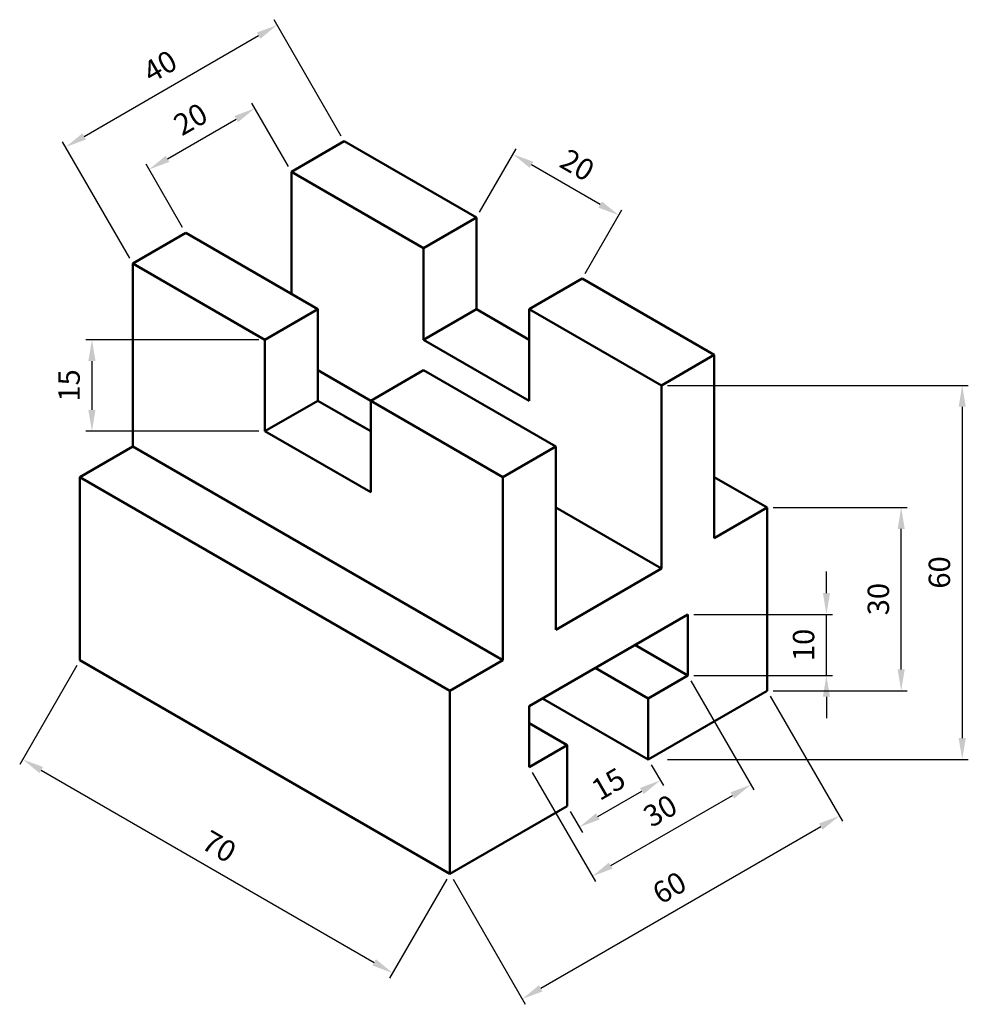
# Model space of a CAD drawing. Units: millimetres. Extents: x 130 to 285, y 54 to 215.
import ezdxf

# ---------------------------------------------------------------- set-up
doc = ezdxf.new("R2010")
doc.units = ezdxf.units.MM
doc.layers.add('M-DIMS', color=3, linetype='Continuous', lineweight=25)
doc.layers.add('M-OUTL', color=7, linetype='Continuous', lineweight=50)
doc.styles.get("Standard").update_dxf_attribs({"font": 'arial.ttf'})
doc.dimstyles.new('AM_ISO$0', dxfattribs={"dimtxt": 3.5, "dimasz": 3.5, "dimexe": 1, "dimexo": 1, "dimgap": 1.5, "dimtad": 1, "dimdsep": 46, "dimtxsty": 'Standard', "dimcen": 0, "dimclrd": 256, "dimclre": 256, "dimclrt": 3, "dimadec": 0, "dimazin": 2, "dimtp": 0.1, "dimtm": 0.1, "dimtfac": 0.71, "dimtmove": 0, "dimatfit": 3, "dimfxl": 1, "dimlwd": -1, "dimlwe": -1, "dimarcsym": 1})

# ---------------------------------------------------------------- blocks, each defined once
blk = doc.blocks.new('*D2')
at = {"layer": 'Defpoints', "color": 0, "transparency": 16777216}
for p in [(239.4, 117.98), (262.11, 117.98), (239.4, 107.98)]:
    blk.add_point(p, dxfattribs=at)
at = {"layer": 'M-DIMS', "color": 0, "linetype": 'ByBlock', "transparency": 16777216}
for p, q in [((262.11, 121.48), (262.11, 124.98)), ((240.4, 117.98), (263.11, 117.98)), ((262.11, 107.98), (262.11, 117.98)), ((240.4, 107.98), (263.11, 107.98)), ((262.11, 104.48), (262.11, 100.98))]:
    blk.add_line(p, q, dxfattribs=at)
at = {"layer": 'M-DIMS', "color": 0, "transparency": 16777216}
for points in [[(261.53, 121.48), (262.69, 121.48), (262.11, 117.98)], [(261.53, 104.48), (262.69, 104.48), (262.11, 107.98)]]:
    blk.add_solid(points, dxfattribs=at)
at = {"layer": 'M-DIMS', "color": 0, "transparency": 16777216, "insert": (258.82, 112.98), "char_height": 3.5, "attachment_point": 5, "rotation": 90}
blk.add_mtext('10', dxfattribs=at)
blk = doc.blocks.new('*D3')
at = {"layer": 'Defpoints', "color": 0, "transparency": 16777216}
for p in [(252.39, 135.48), (274.36, 135.48), (252.39, 105.48)]:
    blk.add_point(p, dxfattribs=at)
at = {"layer": 'M-DIMS', "color": 0, "linetype": 'ByBlock', "transparency": 16777216}
for p, q in [((253.39, 135.48), (275.36, 135.48)), ((274.36, 108.98), (274.36, 131.98)), ((253.39, 105.48), (275.36, 105.48))]:
    blk.add_line(p, q, dxfattribs=at)
at = {"layer": 'M-DIMS', "color": 0, "transparency": 16777216}
for points in [[(273.77, 131.98), (274.94, 131.98), (274.36, 135.48)], [(273.77, 108.98), (274.94, 108.98), (274.36, 105.48)]]:
    blk.add_solid(points, dxfattribs=at)
at = {"layer": 'M-DIMS', "color": 0, "transparency": 16777216, "insert": (271.07, 120.48), "char_height": 3.5, "attachment_point": 5, "rotation": 90}
blk.add_mtext('30', dxfattribs=at)
blk = doc.blocks.new('*D4')
at = {"layer": 'Defpoints', "color": 0, "transparency": 16777216}
for p in [(235.07, 155.48), (235.07, 94.23), (284.36, 94.23)]:
    blk.add_point(p, dxfattribs=at)
at = {"layer": 'M-DIMS', "color": 0, "linetype": 'ByBlock', "transparency": 16777216}
for p, q in [((236.07, 155.48), (285.36, 155.48)), ((284.36, 151.98), (284.36, 97.73)), ((236.07, 94.23), (285.36, 94.23))]:
    blk.add_line(p, q, dxfattribs=at)
at = {"layer": 'M-DIMS', "color": 0, "transparency": 16777216}
for points in [[(283.77, 151.98), (284.94, 151.98), (284.36, 155.48)], [(283.77, 97.73), (284.94, 97.73), (284.36, 94.23)]]:
    blk.add_solid(points, dxfattribs=at)
at = {"layer": 'M-DIMS', "color": 0, "transparency": 16777216, "insert": (281.07, 124.85), "char_height": 3.5, "attachment_point": 5, "rotation": 90}
blk.add_mtext('60', dxfattribs=at)
blk = doc.blocks.new('*D5')
at = {"layer": 'Defpoints', "color": 0, "transparency": 16777216}
for p in [(210.76, 193.37), (204.76, 182.98), (222.08, 172.98)]:
    blk.add_point(p, dxfattribs=at)
at = {"layer": 'M-DIMS', "color": 0, "linetype": 'ByBlock', "transparency": 16777216}
for p, q in [((205.26, 183.84), (211.26, 194.23)), ((225.05, 185.12), (213.79, 191.62)), ((222.58, 173.84), (228.58, 184.23))]:
    blk.add_line(p, q, dxfattribs=at)
at = {"layer": 'M-DIMS', "color": 0, "transparency": 16777216}
for points in [[(214.08, 192.12), (213.5, 191.11), (210.76, 193.37)], [(225.34, 185.62), (224.76, 184.61), (228.08, 183.37)]]:
    blk.add_solid(points, dxfattribs=at)
at = {"layer": 'M-DIMS', "color": 0, "transparency": 16777216, "insert": (221.07, 191.21), "char_height": 3.5, "attachment_point": 5, "rotation": 330}
blk.add_mtext('20', dxfattribs=at)
blk = doc.blocks.new('*D6')
at = {"layer": 'Defpoints', "color": 0, "transparency": 16777216}
for p in [(168.45, 200.87), (174.45, 190.48), (157.13, 180.48)]:
    blk.add_point(p, dxfattribs=at)
at = {"layer": 'M-DIMS', "color": 0, "linetype": 'ByBlock', "transparency": 16777216}
for p, q in [((173.95, 191.34), (167.95, 201.73)), ((154.16, 192.62), (165.42, 199.12)), ((156.63, 181.34), (150.63, 191.73))]:
    blk.add_line(p, q, dxfattribs=at)
at = {"layer": 'M-DIMS', "color": 0, "transparency": 16777216}
for points in [[(165.13, 199.62), (165.71, 198.61), (168.45, 200.87)], [(153.87, 193.12), (154.45, 192.11), (151.13, 190.87)]]:
    blk.add_solid(points, dxfattribs=at)
at = {"layer": 'M-DIMS', "color": 0, "transparency": 16777216, "insert": (158.15, 198.71), "char_height": 3.5, "attachment_point": 5, "rotation": 30}
blk.add_mtext('20', dxfattribs=at)
blk = doc.blocks.new('*D7')
at = {"layer": 'Defpoints', "color": 0, "transparency": 16777216}
for p in [(172.11, 214.53), (183.11, 195.48), (148.47, 175.48)]:
    blk.add_point(p, dxfattribs=at)
at = {"layer": 'M-DIMS', "color": 0, "linetype": 'ByBlock', "transparency": 16777216}
for p, q in [((182.61, 196.34), (171.61, 215.39)), ((140.5, 196.28), (169.08, 212.78)), ((147.97, 176.34), (136.97, 195.39))]:
    blk.add_line(p, q, dxfattribs=at)
at = {"layer": 'M-DIMS', "color": 0, "transparency": 16777216}
for points in [[(168.79, 213.28), (169.37, 212.27), (172.11, 214.53)], [(140.21, 196.78), (140.79, 195.77), (137.47, 194.53)]]:
    blk.add_solid(points, dxfattribs=at)
at = {"layer": 'M-DIMS', "color": 0, "transparency": 16777216, "insert": (153.15, 207.37), "char_height": 3.5, "attachment_point": 5, "rotation": 30}
blk.add_mtext('40', dxfattribs=at)
blk = doc.blocks.new('*D8')
at = {"layer": 'Defpoints', "color": 0, "transparency": 16777216}
for p in [(170.12, 162.98), (141.77, 147.98), (170.12, 147.98)]:
    blk.add_point(p, dxfattribs=at)
at = {"layer": 'M-DIMS', "color": 0, "linetype": 'ByBlock', "transparency": 16777216}
for p, q in [((169.12, 162.98), (140.77, 162.98)), ((141.77, 159.48), (141.77, 151.48)), ((169.12, 147.98), (140.77, 147.98))]:
    blk.add_line(p, q, dxfattribs=at)
at = {"layer": 'M-DIMS', "color": 0, "transparency": 16777216}
for points in [[(141.18, 159.48), (142.35, 159.48), (141.77, 162.98)], [(141.18, 151.48), (142.35, 151.48), (141.77, 147.98)]]:
    blk.add_solid(points, dxfattribs=at)
at = {"layer": 'M-DIMS', "color": 0, "transparency": 16777216, "insert": (138.48, 155.48), "char_height": 3.5, "attachment_point": 5, "rotation": 90}
blk.add_mtext('15', dxfattribs=at)
blk = doc.blocks.new('*D9')
at = {"layer": 'Defpoints', "color": 0, "transparency": 16777216}
for p in [(139.81, 110.48), (200.43, 75.48), (191.05, 59.23)]:
    blk.add_point(p, dxfattribs=at)
at = {"layer": 'M-DIMS', "color": 0, "linetype": 'ByBlock', "transparency": 16777216}
for p, q in [((139.31, 109.61), (129.93, 93.37)), ((133.46, 92.48), (188.02, 60.98)), ((199.93, 74.61), (190.55, 58.37))]:
    blk.add_line(p, q, dxfattribs=at)
at = {"layer": 'M-DIMS', "color": 0, "transparency": 16777216}
for points in [[(133.75, 92.99), (133.17, 91.98), (130.43, 94.23)], [(188.31, 61.49), (187.73, 60.48), (191.05, 59.23)]]:
    blk.add_solid(points, dxfattribs=at)
at = {"layer": 'M-DIMS', "color": 0, "transparency": 16777216, "insert": (162.39, 79.58), "char_height": 3.5, "attachment_point": 5, "rotation": 330}
blk.add_mtext('70', dxfattribs=at)
blk = doc.blocks.new('*D10')
at = {"layer": 'Defpoints', "color": 0, "transparency": 16777216}
for p in [(232.91, 94.23), (234.89, 90.8), (219.64, 86.57)]:
    blk.add_point(p, dxfattribs=at)
at = {"layer": 'M-DIMS', "color": 0, "linetype": 'ByBlock', "transparency": 16777216}
for p, q in [((233.41, 93.36), (235.39, 89.93)), ((224.65, 84.89), (231.85, 89.05)), ((220.14, 85.7), (222.12, 82.28))]:
    blk.add_line(p, q, dxfattribs=at)
at = {"layer": 'M-DIMS', "color": 0, "transparency": 16777216}
for points in [[(231.56, 89.55), (232.15, 88.54), (234.89, 90.8)], [(224.36, 85.4), (224.95, 84.39), (221.62, 83.14)]]:
    blk.add_solid(points, dxfattribs=at)
at = {"layer": 'M-DIMS', "color": 0, "transparency": 16777216, "insert": (226.61, 89.82), "char_height": 3.5, "attachment_point": 5, "rotation": 30}
blk.add_mtext('15', dxfattribs=at)
blk = doc.blocks.new('*D11')
at = {"layer": 'Defpoints', "color": 0, "transparency": 16777216}
for p in [(239.4, 107.98), (213.42, 92.98), (249.73, 90.08)]:
    blk.add_point(p, dxfattribs=at)
at = {"layer": 'M-DIMS', "color": 0, "linetype": 'ByBlock', "transparency": 16777216}
for p, q in [((239.9, 107.11), (250.23, 89.22)), ((213.92, 92.11), (224.25, 74.22)), ((226.78, 76.83), (246.7, 88.33))]:
    blk.add_line(p, q, dxfattribs=at)
at = {"layer": 'M-DIMS', "color": 0, "transparency": 16777216}
for points in [[(246.41, 88.84), (246.99, 87.83), (249.73, 90.08)], [(226.49, 77.34), (227.07, 76.33), (223.75, 75.08)]]:
    blk.add_solid(points, dxfattribs=at)
at = {"layer": 'M-DIMS', "color": 0, "transparency": 16777216, "insert": (235.1, 85.43), "char_height": 3.5, "attachment_point": 5, "rotation": 30}
blk.add_mtext('30', dxfattribs=at)
blk = doc.blocks.new('*D12')
at = {"layer": 'Defpoints', "color": 0, "transparency": 16777216}
for p in [(252.39, 105.48), (264.23, 84.98), (200.43, 75.48)]:
    blk.add_point(p, dxfattribs=at)
at = {"layer": 'M-DIMS', "color": 0, "linetype": 'ByBlock', "transparency": 16777216}
for p, q in [((252.89, 104.61), (264.73, 84.11)), ((215.3, 56.73), (261.2, 83.23)), ((200.93, 74.61), (212.77, 54.11))]:
    blk.add_line(p, q, dxfattribs=at)
at = {"layer": 'M-DIMS', "color": 0, "transparency": 16777216}
for points in [[(260.9, 83.73), (261.49, 82.72), (264.23, 84.98)], [(215, 57.23), (215.59, 56.22), (212.27, 54.98)]]:
    blk.add_solid(points, dxfattribs=at)
at = {"layer": 'M-DIMS', "color": 0, "transparency": 16777216, "insert": (236.6, 72.83), "char_height": 3.5, "attachment_point": 5, "rotation": 30}
blk.add_mtext('60', dxfattribs=at)

msp = doc.modelspace()

# ---------------------------------------------------------------- linework, layer by layer
at = {"layer": 'M-OUTL'}
for p, q in [((174.451, 190.475), (183.111, 195.475)), ((183.111, 195.475), (204.762, 182.975)), ((174.451, 190.475), (196.102, 177.975)), ((174.451, 190.475), (174.451, 170.475)), ((196.102, 177.975), (204.762, 182.975)), ((204.762, 182.975), (204.762, 167.975)), ((148.47, 175.475), (157.13, 180.475)), ((157.13, 180.475), (178.781, 167.975)), ((196.102, 177.975), (196.102, 162.975)), ((148.47, 175.475), (170.121, 162.975)), ((148.47, 175.475), (148.47, 145.475)), ((170.121, 162.975), (148.47, 175.475)), ((213.422, 167.975), (222.082, 172.975)), ((222.082, 172.975), (243.733, 160.475)), ((170.121, 162.975), (178.781, 167.975)), ((178.781, 167.975), (178.781, 152.975)), ((196.102, 162.975), (204.762, 167.975)), ((204.762, 167.975), (213.422, 162.975)), ((213.422, 167.975), (213.422, 152.975)), ((213.422, 167.975), (235.073, 155.475)), ((170.121, 162.975), (170.121, 147.975)), ((196.102, 162.975), (213.422, 152.975)), ((235.073, 155.475), (243.733, 160.475)), ((243.733, 160.475), (243.733, 130.475)), ((187.441, 152.975), (178.781, 157.975)), ((187.441, 152.975), (196.102, 157.975)), ((196.102, 157.975), (217.752, 145.475)), ((235.073, 125.475), (235.073, 155.475)), ((170.121, 147.975), (178.781, 152.975)), ((178.781, 152.975), (187.441, 147.975)), ((187.441, 152.975), (209.092, 140.475)), ((187.441, 152.975), (187.441, 137.975)), ((187.441, 152.975), (209.092, 140.475)), ((209.092, 140.475), (187.441, 152.975)), ((183.111, 150.475), (187.441, 147.975)), ((170.121, 147.975), (187.441, 137.975)), ((148.47, 145.475), (139.81, 140.475)), ((148.47, 145.475), (209.092, 110.475)), ((174.451, 145.475), (187.441, 137.975)), ((209.092, 140.475), (217.752, 145.475)), ((217.752, 145.475), (217.752, 115.475)), ((139.81, 110.475), (139.81, 140.475)), ((139.81, 140.475), (200.432, 105.475)), ((209.092, 110.475), (209.092, 140.475)), ((243.733, 140.475), (252.393, 135.475)), ((217.752, 135.475), (235.073, 125.475)), ((235.073, 125.475), (217.752, 135.475)), ((252.393, 135.475), (243.733, 130.475)), ((252.393, 105.475), (252.393, 135.475)), ((217.752, 115.475), (235.073, 125.475)), ((235.073, 125.475), (217.752, 115.475)), ((213.422, 102.975), (239.403, 117.975)), ((239.403, 107.975), (239.403, 117.975)), ((239.403, 107.975), (230.743, 112.975)), ((200.432, 75.475), (139.81, 110.475)), ((209.092, 110.475), (200.432, 105.475)), ((232.908, 104.225), (224.247, 109.225)), ((232.908, 104.225), (239.403, 107.975)), ((200.432, 105.475), (200.432, 75.475)), ((232.908, 94.225), (252.393, 105.475)), ((232.908, 94.225), (215.587, 104.225)), ((232.908, 94.225), (232.908, 104.225)), ((213.422, 92.975), (213.422, 102.975)), ((219.645, 96.568), (213.422, 100.161)), ((213.422, 92.975), (219.645, 96.568)), ((219.645, 86.568), (219.645, 96.568)), ((200.432, 75.475), (219.645, 86.568))]:
    msp.add_line(p, q, dxfattribs=at)

# ---------------------------------------------------------------- dimensions: what is measured, and where the dimension line sits
at = {"layer": 'M-DIMS'}
for p1, p2, distance, override, picture, middle in [((148.47, 175.475), (183.111, 195.475), 22, {"dimclrd": 0, "dimclre": 0, "dimclrt": 0}, '*D7', (153.147, 207.375)), ((157.13, 180.475), (174.451, 190.475), 12, {"dimclrd": 0, "dimclre": 0, "dimclrt": 0}, '*D6', (158.147, 198.714)), ((222.082, 172.975), (204.762, 182.975), -12, {"dimclrd": 0, "dimclre": 0, "dimclrt": 0}, '*D5', (221.066, 191.214)), ((170.121, 162.975), (170.121, 147.975), -28.353, {"dimclrd": 0, "dimclre": 0, "dimclrt": 0}, '*D8', (138.481, 155.475)), ((252.393, 105.475), (252.393, 135.475), -21.964, {"dimpost": '', "dimclrd": 0, "dimclre": 0, "dimclrt": 0}, '*D3', (271.069, 120.475)), ((239.403, 107.975), (239.403, 117.975), -22.706, {"dimpost": '', "dimclrd": 0, "dimclre": 0, "dimclrt": 0}, '*D2', (258.822, 112.975)), ((139.81, 110.475), (200.432, 75.475), -18.756, {"dimclrd": 0, "dimclre": 0, "dimclrt": 0}, '*D9', (162.386, 79.579)), ((213.422, 92.975), (239.403, 107.975), -20.66, {"dimclrd": 0, "dimclre": 0, "dimclrt": 0}, '*D11', (235.098, 85.431)), ((200.432, 75.475), (252.393, 105.475), -23.667, {"dimclrd": 0, "dimclre": 0, "dimclrt": 0}, '*D12', (236.603, 72.825))]:
    dim = msp.add_aligned_dim(p1=p1, p2=p2, distance=distance, dimstyle='AM_ISO$0', override=override, dxfattribs=at)
    dim.commit()
    dim.dimension.update_dxf_attribs({"geometry": picture, "text_midpoint": middle})
for p1, p2, distance, text, picture, middle in [((235.073, 155.475), (235.073, 94.225), 49.285, '60', '*D4', (281.07, 124.85)), ((219.645, 86.568), (232.908, 94.225), -3.957, '15', '*D10', (226.611, 89.817))]:
    dim = msp.add_aligned_dim(p1=p1, p2=p2, distance=distance, text=text, dimstyle='AM_ISO$0', override={"dimpost": '', "dimclrd": 0, "dimclre": 0, "dimclrt": 0}, dxfattribs=at)
    dim.commit()
    dim.dimension.update_dxf_attribs({"geometry": picture, "text_midpoint": middle})

doc.saveas('drawing.dxf')
